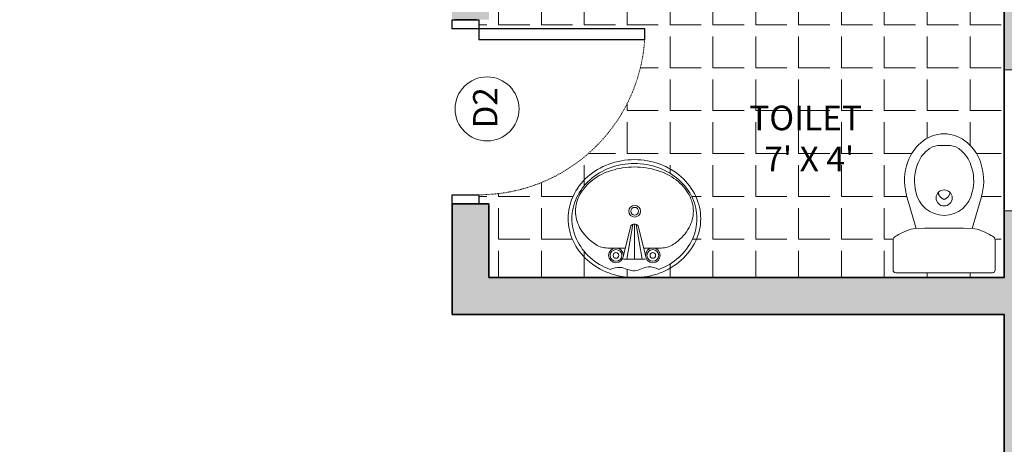
# Model space of a CAD drawing. Units: inches. Extents: x 2701 to 6846, y 811 to 2447.
# Tile 14 of 20: x 2926 to 3086, y 1231 to 1300. Entities that reach past the tile are written whole.
import ezdxf

# ---------------------------------------------------------------- set-up
doc = ezdxf.new("R2010")
doc.units = ezdxf.units.IN
doc.linetypes.add('HIDDEN4', pattern=[0.09375, 0.0625, -0.03125])
for name, color, linetype, lineweight in [('A-ANNO-IDEN', 7, 'Continuous', 13), ('A-AREA-IDEN', 7, 'Continuous', 18), ('A-DOOR', 4, 'Continuous', 25), ('A-DOOR-SWNG', 4, 'HIDDEN4', 13), ('A-FLOR-FIXT', 7, 'Continuous', 18), ('A-FLOR-PATT', 252, 'Continuous', 13), ('A-GLAZ', 4, 'Continuous', 18), ('A-WALL', 7, 'Continuous', 35)]:
    doc.layers.add(name, color=color, linetype=linetype, lineweight=lineweight)
doc.layers.add('A-WALL-PATT', color=18, linetype='Continuous', lineweight=13, true_color=0x000000)
doc.styles.get("Standard").update_dxf_attribs({"font": 'arial.ttf'})

# ---------------------------------------------------------------- blocks, each defined once
blk = doc.blocks.new('V')
for p, q in [((3304.149234297809, 1279.327014385662), (3281.149234297809, 1279.327014385662)), ((3304.149234297809, 1277.327014385662), (3281.149234297809, 1277.327014385662)), ((3304.149234297809, 1275.327014385662), (3281.149234297809, 1275.327014385662)), ((3281.149234297809, 1273.327014385662), (3304.149234297809, 1273.327014385662))]:
    blk.add_line(p, q)
blk.add_circle((3293.674463800009, 1283.693074863908), 3.189132293142032)
at = {"insert": (3292.450488040435, 1284.761898613762), "char_height": 2.5, "attachment_point": 1}
blk.add_mtext_dynamic_manual_height_columns('V', width=0.0152702913619578, gutter_width=12.5, heights=[0], dxfattribs=at)
blk = doc.blocks.new('V1')
for p, q in [((3281.149234297809, 1279.327014385662), (3281.149234297809, 1273.327014385662)), ((3304.149234297809, 1273.327014385662), (3304.149234297809, 1279.327014385662))]:
    blk.add_line(p, q)
blk.add_blockref('V', (0, 0))
blk = doc.blocks.new('A$C62EA08CE')
at = {"linetype": 'ByBlock'}
for p, q in [((0.2190750854661019, 0.3943350335612194), (0.306705085467911, 0.3943350335612194)), ((0.2328389724007138, 0.3943350335612194), (0.256592247476874, 0.2566437564746593)), ((0.2628900854706444, 0.3943350335612194), (0.2628900854706444, 0.2555161210839287)), ((0.2933077018988115, 0.3943350335612194), (0.2695802776597702, 0.256794098582759)), ((0.2190750854661019, 0.3797300335645559), (0.2482850854667049, 0.2628900335621438)), ((0.2774950854673079, 0.2628900335621438), (0.306705085467911, 0.3797300335645559)), ((0.1569030901755468, 0.3505200335639529), (0.2263775854680716, 0.3505200335639529)), ((0.2994025854659412, 0.3505200335639529), (0.3690778702966782, 0.3505200335639529))]:
    blk.add_line(p, q, dxfattribs=at)
for centre, radius in [((0.1898650854727748, 0.3797300335645559), 0.02921), ((0.1898650854727748, 0.3797300335645559), 0.02321), ((0.1898650854727748, 0.3797300335645559), 0.01121), ((0.335915085468514, 0.3797300335645559), 0.02921), ((0.335915085468514, 0.3797300335645559), 0.02321), ((0.335915085468514, 0.3797300335645559), 0.01121), ((0.2640384579517558, 0.2045255693010404), 0.023368), ((0.2640384579517558, 0.2045255693010404), 0.015368)]:
    blk.add_circle(centre, radius, dxfattribs=at)
for centre, radius, start, end in [((0.2518357941607974, 0.202225176646607), 0.2631644933429036, 110.2132031902237, 131.6335499305747), ((0.2518357941607974, 0.202225176646607), 0.2481644933429036, 110.2132031902237, 131.6335499305747), ((0.2628901093212335, 0.172201390065311), 0.2951586434963838, 90.00000458569829, 110.2131769401282), ((0.2628900616127794, 0.172201390065311), 0.2951586434963838, 69.78682305987175, 89.9999954143017), ((0.2739443767732155, 0.202225176646607), 0.2481644933429035, 48.36645006942531, 69.78679680977629), ((0.2739443767732155, 0.202225176646607), 0.2631644933429035, 48.36645006942531, 69.78679680977629), ((0.2348020259832992, 0.2213881285715615), 0.2375253048786466, 131.6335451873388, 155.0149376704166), ((0.2909781449579896, 0.2213881285715615), 0.2375253048786464, 24.98506232958336, 48.36645481266113), ((0.2348020259832992, 0.2213881285715615), 0.2225253048786466, 131.6335451873388, 155.0149376704166), ((0.2909781449579896, 0.2213881285715615), 0.2225253048786464, 24.98506232958336, 48.36645481266113), ((0.2084237233957538, 0.23368008415855), 0.208423637924446, 155.0149182782628, 180.0000137570949), ((0.2084237233957538, 0.23368008415855), 0.1934236379244461, 155.0149182782628, 180.0000137570949), ((0.2106628391502454, 0.177718259532412), 0.18834914705, 122.2598079089317, 151.0887990604045), ((0.1569030901755468, 0.2628900335621438), 0.08763, 90, 122.2598079089317), ((0.3690778702966782, 0.2628900335621438), 0.08763, 56.09549019404326, 90), ((0.2835224813406967, 0.1355918312110589), 0.24100718245, 53.1301018541481, 56.09549019404326), ((0.3151173317910434, 0.177718259532412), 0.18834914705, 28.91120093959547, 53.1301018541481), ((0.317356447545535, 0.23368008415855), 0.1934236379244455, 359.9999862429051, 24.98508172173719), ((0.317356447545535, 0.23368008415855), 0.2084236379244456, 359.9999862429051, 24.98508172173719), ((0.1622244803456851, 0.2044700335609377), 0.13301439488, 151.0887990604045, 180), ((0.2628900854706444, 0.2736666355558555), 0.018150514468869, 216.4225302188404, 323.5774697811596), ((0.3635556905883277, 0.2044700335609377), 0.13301439488, 0, 28.91120093959547), ((0.2084237233957538, 0.2336799829718075), 0.2084236379244456, 179.9999862429051, 204.9850817217372), ((0.2084237233957538, 0.2336799829718075), 0.1934236379244455, 179.9999862429051, 204.9850817217372), ((0.1622244803456851, 0.2044700335609377), 0.13301439488, 180, 208.9112009395955), ((0.3635556905883277, 0.2044700335609377), 0.13301439488, 331.0887990604045, 0), ((0.317356447545535, 0.2336799829718075), 0.1934236379244461, 335.0149182782628, 1.37570948859e-05), ((0.317356447545535, 0.2336799829718075), 0.208423637924446, 335.0149182782628, 1.37570948859e-05), ((0.2348020259832992, 0.2459719385587959), 0.2375253048786464, 204.9850623295834, 228.3664548126612), ((0.2348020259832992, 0.2459719385587959), 0.2225253048786464, 204.9850623295834, 228.3664548126612), ((0.2106628391502454, 0.2312218075967394), 0.18834914705, 208.9112009395955, 233.1301018541481), ((0.3151173317910434, 0.2312218075967394), 0.18834914705, 306.8698981458519, 331.0887990604045), ((0.2909781449579896, 0.2459719385587959), 0.2225253048786466, 311.6335451873388, 335.0149376704167), ((0.2909781449579896, 0.2459719385587959), 0.2375253048786466, 311.6335451873388, 335.0149376704167), ((0.2518357941607974, 0.2651348904837505), 0.2481644933429134, 228.3664500694253, 249.7867968097763), ((0.2422576896005921, 0.2733482359108166), 0.24100718245, 233.1301018541481, 252.7420607856108), ((0.2835224813406967, 0.2733482359108166), 0.24100718245, 287.2579392143892, 306.8698981458519), ((0.2739443767732155, 0.2651348904837505), 0.2481644933429136, 290.2132031902237, 311.6335499305747), ((0.2518357941607974, 0.2651348904837505), 0.2631644933429134, 228.3664500694253, 249.7867968097763), ((0.2628900854706444, 0.3397629544924712), 0.31055292093, 252.7420607856108, 270), ((0.2628900854706444, 0.3397629544924712), 0.31055292093, 270, 287.2579392143892), ((0.2739443767732155, 0.2651348904837505), 0.2631644933429136, 290.2132031902237, 311.6335499305747), ((0.2628901093212335, 0.2951586770577705), 0.2951586434963766, 249.7868230598717, 269.9999954143017), ((0.2628901093212335, 0.2951586770577705), 0.2801586434963766, 249.7868230598717, 269.9999954143017), ((0.2628900616127794, 0.2951586770577705), 0.2801586434963765, 270.0000045856983, 290.2131769401283), ((0.2628900616127794, 0.2951586770577705), 0.2951586434963765, 270.0000045856983, 290.2131769401283)]:
    blk.add_arc(centre, radius, start, end, dxfattribs=at)
blk.add_open_spline([(0.1660913743126002, 0.4351060694243643), (0.1795429390761559, 0.4305676737460202), (0.2123752678413389, 0.4194904420932696), (0.2631088802261481, 0.454314446693237), (0.3131553959096029, 0.4161820139975771), (0.3454695139184305, 0.4293234167515693), (0.3596887966214126, 0.4351060694243643)], degree=3, knots=[0, 0, 0, 0, 0.0411087303528805, 0.1003374234737184, 0.1559132068848227, 0.1995857666183122, 0.1995857666183122, 0.1995857666183122, 0.1995857666183122], dxfattribs=at)
blk = doc.blocks.new('A$C150B42AD')
at = {"ltscale": 20}
for p, q in [((0.2429999219411911, 0.6605010896237218), (0.0124999219360689, 0.6605010896237218)), ((0.2429999219411911, 0.6605010896237218), (0.4734999219390375, 0.6605010896237218)), ((-7.80610208e-08, 0.6480010896266322), (-7.80610208e-08, 0.5079979540751083)), ((0.4859999219361271, 0.6480010896266322), (0.4859999219361271, 0.5079979540751083)), ((0.1099663932354815, 0.4499086118448759), (0.0669662435202554, 0.3038111749119707)), ((0.1071200985052201, 0.4500080066427472), (0.1510932948976915, 0.4484724287904101)), ((0.1510932948976915, 0.4484724287904101), (0.2429999219411911, 0.4484724287904101)), ((0.3349065489774148, 0.4484724287904101), (0.2429999219411911, 0.4484724287904101)), ((0.3788797453698862, 0.4500080066427472), (0.3349065489774148, 0.4484724287904101)), ((0.3760334506469007, 0.4499086118448759), (0.419033600354851, 0.3038111749119707)), ((0.2244999219356032, 0.0549026304142899), (0.2429999219411911, 0.0549026304142899)), ((0.2614999219395031, 0.0549026304142899), (0.2429999219411911, 0.0549026304142899))]:
    blk.add_line(p, q, dxfattribs=at)
for centre, radius, start, end in [((0.0124999219360689, 0.6480010896266322), 0.0125, 90, 180), ((0.4734999219390375, 0.6480010896266322), 0.0125, 0, 90), ((0.0239999219365927, 0.5079979540751083), 0.024, 180, 243.9999999999169), ((0.2288323805723849, 0.861211124320107), 0.4322502624564528, 240.1180548737387, 247.8819451258213), ((0.2571674633099974, 0.861211124320107), 0.4322502624564528, 292.1180548741787, 299.8819451262613), ((0.4619999219385136, 0.5079979540751083), 0.024, 296.0000000000832, 0), ((0.1119175659141547, 0.5519209073245293), 0.1020257566424159, 243.3048371366711, 267.3048371363805), ((0.3740822779682276, 0.5519209073245293), 0.1020257566424159, 272.6951628636196, 296.6951628633288), ((0.2429999219411911, 0.2520000365038868), 0.1359999999999445, 90, 170.1093554438925), ((0.2429999219411911, 0.2520000365038868), 0.1359999999999054, 9.890644556107487, 90), ((0.2429999219411911, 0.3047433868632652), 0.0383668793900662, 90, 270), ((0.2429999219411911, 0.3047433868632652), 0.0383668793900662, 270, 90), ((0.3111168528876078, 0.2222454825459863), 0.2564589547706602, 165.7117968948095, 200.3376824053133), ((0.2429999219411911, 0.2520000365038868), 0.1834999999995578, 163.5995179369745, 169.4685073238174), ((0.2251027765405524, 0.2821865844234708), 0.0095725464836317, 149.1844377639907, 231.8077122469979), ((0.2644505607122483, 0.2649244167114375), 0.0524797911919514, 119.1738126186074, 155.015614861567), ((0.2438841986540865, 0.2978098350213258), 0.0138752344263254, 93.65396949145695, 111.1904535314196), ((0.2421156452282958, 0.2978098350213258), 0.0138752344263254, 68.80954646858042, 86.34603050854304), ((0.221549283162858, 0.2649244167114375), 0.0524797911919514, 24.98438513843297, 60.82618738139257), ((0.2608970673345539, 0.2821865844234708), 0.0095725464836317, 308.1922877530021, 30.81556223600924), ((0.1748829909874985, 0.2222454825459863), 0.2564589547707392, 339.6623175946867, 14.28820310476077), ((0.2429999219411911, 0.2520000365038868), 0.1834999999998773, 10.53149267661153, 16.40048206346955), ((0.3111168528876078, 0.2222454825459863), 0.2089589547707847, 165.2744742501726, 200.6077610261089), ((0.1748829909874985, 0.2222454825459863), 0.2089589547707847, 339.3922389738912, 14.72552574982734), ((0.2579999219406091, 0.1940000364993466), 0.1494999999998057, 197.6390904734559, 230.6281882087223), ((0.2279999219417732, 0.1940000364993466), 0.1494999999996299, 309.3718117912777, 342.360909526544), ((0.2579999219406091, 0.1940000364993466), 0.1969999999999626, 198.0034048038204, 230.2740437647753), ((0.2279999219417732, 0.1940000364993466), 0.1969999999999626, 309.7259562352247, 341.9965951961797), ((0.2429999219411911, 0.1660000365009182), 0.1184999999993879, 227.6454679706322, 235.8467474759224), ((0.2244999219356032, 0.149902630415454), 0.0949999999999961, 239.6323803004523, 270), ((0.2614999219395031, 0.149902630415454), 0.0949999999999961, 270, 300.3676196995477), ((0.2429999219411911, 0.1660000365009182), 0.1185000000000767, 304.1532525240776, 312.3545320293678), ((0.2429999219411911, 0.1660000365009182), 0.1660000000001673, 228.0788004750028, 270), ((0.2429999219411911, 0.1660000365009182), 0.16599999999994, 270, 311.9211995251523)]:
    blk.add_arc(centre, radius, start, end, dxfattribs=at)
blk = doc.blocks.new('DOOR-D2-30IN-PANEL-FRAME')
blk.add_lwpolyline([(-4.547e-13, 30.00000000000046), (-4.547e-13, 28.52062868157645), (4.3614931230818, 28.52062868157645), (4.3614931230818, 30.00000000000046), (-4.547e-13, 30.00000000000046)], close=True)
for points in [[(3.925343810773938, 30.00000000000046), (0.4361493129576957, 30.00000000000046)], [(4.361493123406944, 0), (4.361493123406944, 3.223968567697738), (31.40275048651847, 3.22396856790101), (31.40275048651847, 1.479371318667745), (1.623448e-10, 1.479371318424), (1.623448e-10, 0)], [(1.623448e-10, 0), (4.361493123406944, 0)], [(3.925343810773938, 0), (0.4361493129576957, 0)]]:
    blk.add_lwpolyline(points)

msp = doc.modelspace()

# ---------------------------------------------------------------- hatches: boundary and pattern name
at = {"layer": 'A-FLOR-PATT'}
h = msp.add_hatch(dxfattribs=at)
h.set_pattern_fill('ANGLE', color=256)
h.set_pattern_definition([(0, (0, 0), (0, 6.985), [5.08, -1.905]), (90, (0, 0), (-6.985, 4e-16), [5.08, -1.905])])
h.paths.add_polyline_path([(2841.812531618507, 1296.510714093028, -0.1094531397224823), (2842.614165366529, 1300.128842847245, -0.1023747835315324), (2844.977063233859, 1303.301704019213, -0.0937428406070795), (2848.425874088265, 1305.367635711971, -0.0624630522953803), (2851.366818664733, 1306.050044742079), (2785.971391037217, 1306.050044742079), (2785.971391037217, 1258.050044742079), (2827.971391037217, 1258.050044742079), (2827.971391037217, 1256.411537864998), (2829.450762355621, 1256.411537864998, -0.3948265708167148), (2854.747422469505, 1283.452795228435), (2856.49201971855, 1283.452795228435), (2856.49201971876, 1256.411537865324), (2857.971391037219, 1256.411537865324), (2857.971391037219, 1258.05004474208), (2863.971391037218, 1258.050044742079), (2863.971391037217, 1306.050044742079), (2853.867060923166, 1306.050044742079, -0.0624630504647152), (2856.808005416599, 1305.367635742541, -0.0937428427235612), (2860.256816355725, 1303.301704017657, -0.1023747714125829), (2862.619714024758, 1300.128843269809, -0.1094531521575188), (2863.421347969692, 1296.510714138194, -0.109453153989093), (2862.619714017641, 1292.892584946142, -0.1023747709767553), (2860.256816355757, 1289.719724213534, -0.093738257087872), (2856.808189965141, 1287.653860434733, -0.0884250558281599), (2852.616939784454, 1286.906795737127, -0.0884250554332989), (2848.425689622791, 1287.653860434813, -0.0937382570330623), (2844.977063234018, 1289.719724212192, -0.1023747824199799), (2842.614165384649, 1292.892585345091, -0.1094531396555831)])
h.paths.add_polyline_path([(2805.214857085719, 1273.877134568363, -0.141745245190178), (2808.318689175414, 1271.772621468736, -0.1849834247598648), (2809.773740825251, 1267.974277286972, -0.1849834247688995), (2808.318689175285, 1264.175933105053, -0.141745244968364), (2805.214857091107, 1262.071420007333, -0.1522440861962393), (2799.994488829542, 1261.79557176336, -0.0256138964539793), (2799.368711507224, 1261.94541476925), (2794.365115778627, 1263.418098821323), (2794.36467071784, 1263.405353947873, -0.1112416791490392), (2793.99312620013, 1261.915170284834, -0.0338893268367682), (2793.114424873909, 1260.113565580275, -0.286745385218), (2792.375651823606, 1259.651928944151), (2787.580775843661, 1259.651928944133, -0.4142135623681101), (2787.152671505053, 1260.080033282747), (2787.152671505153, 1267.974277286972), (2787.152671505053, 1275.868521290948, -0.4142135623730951), (2787.580775843668, 1276.296625629562), (2792.375651823623, 1276.296625629544, -0.2867453846084762), (2793.114424873105, 1275.834988995069, -0.0338893268640583), (2793.99312620013, 1274.033384289111, -0.1051042356073151), (2794.361711671137, 1272.627936636842), (2794.365115778619, 1272.530455752619), (2799.368711507498, 1274.003139804786, -0.0256138965941945), (2799.994488833287, 1274.152982811292, -0.1522440859162748)], flags=16)
h.paths.add_polyline_path([(2804.681063364808, 1272.339952816459, -0.1449445299175104), (2807.087654609562, 1270.708506585421, -0.0358001151589041), (2807.447023191777, 1270.252713401882, -0.1332846890906797), (2807.893417732773, 1268.607871708063), (2807.893417732813, 1267.974277286972), (2807.893417732773, 1267.340682865632, -0.1332846888970446), (2807.447023193029, 1265.695841173949, -0.0358001152638917), (2807.087654609923, 1265.240047988954, -0.1449445297267833), (2804.681063368992, 1263.608601758809, -0.1554037438169349), (2800.343099481134, 1263.385728797012, -0.3645106918446579), (2796.485382154562, 1267.974277286972, -0.3645106920174053), (2800.343099483932, 1272.562825777418, -0.1554037435534987)], flags=0)
h.paths.add_polyline_path([(2800.015880108981, 1268.901471623875, 0.1692977046764319), (2799.131174998024, 1268.11576383613, 0.0766670309700064), (2799.100009657075, 1267.974277286936, 0.0766670313951798), (2799.13117499834, 1267.832790736999, 0.1692977045836763), (2800.015880108981, 1267.04708294982, 0.3052192884941762), (2800.365297210358, 1267.156497374013, 0.1695347489604994), (2800.650786991011, 1267.974277286972, 0.1695347391656343), (2800.365297241503, 1268.792057160761, 0.3052193300480048)], flags=0)
h.paths.add_polyline_path([(2971.971391037218, 1456.050044742079), (2923.971391037218, 1456.050044742079), (2923.971391037218, 1408.050044742079), (2922.332884160136, 1408.050044742079), (2922.332884160136, 1406.570673423676, -0.394826570816717), (2949.374141523573, 1381.274013309792), (2949.374141523573, 1379.529416060747), (2922.332884160461, 1379.529416060537), (2922.332884160461, 1378.050044742079), (2923.971391037218, 1378.050044742079), (2923.971391037217, 1372.050044742079), (2971.971391037217, 1372.050044742079)])
h.paths.add_polyline_path([(2939.8177624336, 1436.526417411941, -0.1417452451905352), (2937.713249333971, 1433.422585322236, -0.1849834247599418), (2933.914905152205, 1431.967533672398, -0.1849834247691276), (2930.116560970283, 1433.422585322367, -0.1417452449676952), (2928.01204787257, 1436.526417406529, -0.1522440861964963), (2927.736199628592, 1441.746785668103, -0.0256138964540868), (2927.886042634483, 1442.372562990423), (2929.358726686557, 1447.376158719022), (2929.345981813088, 1447.376603779809, -0.1112416791473441), (2927.855798150072, 1447.748148297517, -0.0338893268369074), (2926.054193445506, 1448.626849623741, -0.2867453852169366), (2925.592556809384, 1449.365622674043), (2925.592556809366, 1454.160498653989, -0.4142135623681173), (2926.020661147981, 1454.588602992596), (2933.914905152205, 1454.588602992496), (2941.809149156182, 1454.588602992596, -0.4142072303161659), (2942.237253494696, 1454.160507909187), (2942.237253494777, 1449.365622674043, -0.2867453846243844), (2941.775616860276, 1448.626849624529, -0.0338893268635044), (2939.974012154347, 1447.74814829752, -0.1051042356087532), (2938.568564502058, 1447.379562826511), (2938.471083617852, 1447.37615871903), (2939.943767670019, 1442.372562990154, -0.0256138965942444), (2940.093610676525, 1441.746785664364, -0.152244085915992)], flags=16)
h.paths.add_polyline_path([(2938.280580681695, 1437.060211132847, -0.1449445299182329), (2936.649134450649, 1434.653619888082, -0.0358001151583613), (2936.193341267117, 1434.294251305872, -0.1332846890907526), (2934.548499573297, 1433.847856764876), (2933.914905152205, 1433.847856764836), (2933.281310730865, 1433.847856764876, -0.1332846888976268), (2931.636469039176, 1434.294251304624, -0.0358001152630847), (2931.180675854191, 1434.653619887722, -0.14494452972667), (2929.549229624045, 1437.06021112865, -0.1554037438170702), (2929.326356662246, 1441.398175016512, -0.3645106918448713), (2933.914905152205, 1445.255892343087, -0.3645106920173691), (2938.503453642651, 1441.398175013717, -0.1554037435532691)], flags=0)
h.paths.add_polyline_path([(2969.158462562638, 1392.044508285666, -0.0937428443921736), (2971.224394311477, 1388.595697278927, -0.0884209696484748), (2971.971391037217, 1384.404631716083, -0.0884209680179829), (2971.224394332037, 1380.213566228077, -0.0937428458331012), (2969.158462561081, 1376.764755163806, -0.1023747798731684), (2965.985601516888, 1374.401857356678, -0.1094531425013952), (2962.367472681615, 1373.600223549837, -0.1094531553411192), (2958.74934344807, 1374.401857521223, -0.102374769792102), (2955.576482756955, 1376.764755163771, -0.0937382570879047), (2953.510618978154, 1380.213381554388, -0.0884250558281564), (2952.763554280548, 1384.404631735075, -0.0884250554336261), (2953.510618978239, 1388.595881896752, -0.0937382570324601), (2955.576482755607, 1392.044508285504, -0.1023747638736991), (2958.749343238892, 1394.40740583216, -0.10945316082308), (2962.367472636449, 1395.209039901022, -0.1094531494878097), (2965.985601690358, 1394.407406013345, -0.102374774975509)], flags=0)
edge = h.paths.add_edge_path(flags=16)
edge.add_arc((2961.074722408913, 1384.858947505427), 10.19921062335061, 20.21320321302568, 41.63359467655653, ccw=False)
edge.add_spline(control_points=[(2970.645798607602, 1388.382922212802), (2970.45927694694, 1387.830081875375), (2970.004018351208, 1386.480719475378), (2971.435235818619, 1384.395639569603), (2969.86804662324, 1382.338798369057), (2970.408139739579, 1381.010733700175), (2970.645798607602, 1380.426341238356)], knot_values=[0, 0, 0, 0, 0.0411087303528805, 0.1003374234737184, 0.1559132068848227, 0.1995857666183122, 0.1995857666183122, 0.1995857666183122, 0.1995857666183122], degree=3, periodic=0)
edge.add_arc((2961.074722408954, 1383.950315945844), 10.19921062335061, 318.3664053106646, 339.7867967863075, ccw=False)
edge.add_arc((2961.862292702369, 1383.250252100635), 9.145476143303874, 294.98529005245234, 318.3664053112933, ccw=False)
edge.add_arc((2962.367474738348, 1382.166141072693), 7.949438681384353, 269.9999862429006, 294.9853451035073, ccw=False)
edge.add_arc((2962.367470579714, 1382.166141072693), 7.949438681384465, 245.0146528606722, 270.00001621636034, ccw=False)
edge.add_arc((2962.872652615592, 1383.250252100682), 9.145476143303885, 221.633594689284, 245.0147081786685, ccw=False)
edge.add_arc((2963.660222908995, 1383.950315945905), 10.19921062335051, 200.2129623510071, 221.6335946899624, ccw=False)
edge.add_arc((2964.894158186733, 1384.404632705954), 11.5141250647146, 180.0000045856949, 200.2129623497761, ccw=False)
edge.add_arc((2964.894158186734, 1384.404630744956), 11.51412506471477, 159.7870376490639, 179.999994827515, ccw=False)
edge.add_arc((2963.660222908922, 1384.858947504804), 10.19921062335051, 138.3664053200289, 159.7870376464858, ccw=False)
edge.add_arc((2962.872652615694, 1385.559011350224), 9.145476143303881, 114.9852895697228, 138.3664053235114, ccw=False)
edge.add_arc((2962.367470579715, 1386.643122378167), 7.949438681384341, 89.99998624290072, 114.9853445481478, ccw=False)
edge.add_arc((2962.367474738348, 1386.643122378167), 7.949438681384461, 65.01465414332972, 90.00001621635698, ccw=False)
edge.add_arc((2961.862292702924, 1385.559011349966), 9.145476143303876, 41.63359468007258, 65.01470929671348, ccw=False)
h.paths.add_polyline_path([(2963.809881193461, 1393.327235568244, -0.1264579126559968), (2966.613496696745, 1390.682864813822, -0.1416969839114421), (2967.169431848072, 1388.76054773013), (2967.169431848171, 1387.405856218539, -1), (2969.570411442753, 1387.40585621857, -0.4142135626407067), (2968.369921644365, 1386.205366421279), (2963.567962456663, 1385.004876624353, 0.146217798515541), (2963.311249278865, 1384.663463983469), (2968.97016654397, 1385.639690083447), (2968.97016654397, 1383.154510596366), (2963.317428127216, 1384.129674263443, 0.1403115373898127), (2963.56796245605, 1383.804386826958), (2968.369921645561, 1382.603897029581, -0.4142135623489124), (2969.570411442753, 1381.403407232289, -1), (2967.169431848171, 1381.403407232289), (2967.169431848072, 1380.040463554169, -0.1490250791000606), (2966.557068512987, 1378.031526062613, -0.0127594246128423), (2966.264512020975, 1377.619349736432, -0.1063032105074506), (2963.809880694587, 1375.482028786924, -0.1268223860120219), (2961.166982861567, 1374.800713347196, -0.12682239841106), (2958.52408452876, 1375.482027883284, -0.1063031789236789), (2956.069454414507, 1377.619348785205, -0.0857220920089208), (2954.537253221299, 1380.622635309784, -0.0753510219692474), (2953.964044077883, 1384.404631725429, -0.0753510220208753), (2954.537253222076, 1388.186628143578, -0.0857220919249397), (2956.069454414099, 1391.189914665108, -0.1063031717113424), (2958.5240850283, 1393.327234664099, -0.1268223860250843), (2961.166982861567, 1394.008550103962, -0.1268223983642548)], flags=0)
h.paths.add_polyline_path([(2934.842099489099, 1441.725394388693, 0.1692977046741335), (2934.056391701355, 1442.610099499628, 0.0766670309649834), (2933.91490515217, 1442.641264840574, 0.0766670314095982), (2933.773418602207, 1442.610099499295, 0.1692977045780331), (2932.987710815057, 1441.72539438868, 0.305219290057435), (2933.097125240708, 1441.375977286128, 0.169534748594888), (2933.914905152205, 1441.090487506638, 0.1695347390414705), (2934.732685025499, 1441.375977255749, 0.3052193305973386)], flags=0)
h.paths.add_polyline_path([(2969.323819906164, 1387.40585621857, -1), (2967.416023384759, 1387.40585621857, -1)], flags=0)
h.paths.add_polyline_path([(2968.830636832988, 1387.40585621857, -1), (2967.909206457936, 1387.40585621857, -1)], flags=0)
h.paths.add_polyline_path([(2962.129657139981, 1384.357435236314, -1), (2960.208873464314, 1384.357435236314, -1)], flags=0)
h.paths.add_polyline_path([(2961.800868424529, 1384.357435236314, -1), (2960.537662179766, 1384.357435236314, -1)], flags=0)
h.paths.add_polyline_path([(2969.323819906164, 1381.403407232289, -1), (2967.416023384759, 1381.403407232289, -1)], flags=0)
h.paths.add_polyline_path([(2968.830636832988, 1381.403407232289, -1), (2967.909206457936, 1381.403407232289, -1)], flags=0)
h.paths.add_polyline_path([(3085.971391037217, 1306.050044742079), (3001.971391037217, 1306.050044742079), (3001.971391037217, 1300.050044742079), (3000.332884160462, 1300.050044742079), (3000.332884160462, 1298.570673423621), (3027.374141523574, 1298.570673423411), (3027.374141523574, 1296.826076174374, -0.3948265708167921), (3000.332884160137, 1271.529416060482), (3000.332884160137, 1270.050044742079), (3001.971391037216, 1270.050044742079), (3001.971391037217, 1258.050044742079), (3085.971391037217, 1258.050044742079)])
h.paths.add_polyline_path([(3033.332715044416, 1274.444953022308, -0.1023747723857111), (3035.695612729331, 1271.272092240373, -0.1094531510467398), (3036.49724665838, 1267.653963142847, -0.109453129065687), (3035.695613062762, 1264.035834715682, -0.102374792813879), (3033.332715044451, 1260.862973218194, -0.0937428491083937), (3029.883903848349, 1258.797041398739, -0.0884209654955001), (3025.692838473141, 1258.05004474208, -0.0884209669723455), (3021.501773032378, 1258.797041429867, -0.093742846952782), (3018.052961922706, 1260.862973216846, -0.1023747779170817), (3015.690064146835, 1264.035834192024, -0.1094531447948728), (3014.888430307195, 1267.653963097683, -0.1094531229044609), (3015.690063814699, 1271.272091335764, -0.1023747982671114), (3018.052961922546, 1274.444953023867, -0.0937382570344717), (3021.501588311451, 1276.510816801145, -0.0884250558280669), (3025.692838492134, 1277.25788149875, -0.0884250554332868), (3029.884088653796, 1276.510816801064, -0.0937382570874262)], flags=0)
edge = h.paths.add_edge_path(flags=16)
edge.add_arc((3026.847218107582, 1267.148783163603), 9.145476143303444, 24.985288685417686, 48.36640531129461, ccw=False)
edge.add_arc((3027.931329135525, 1267.653965199581), 7.949438681383711, -1.3757099395661498e-05, 24.98534353079839, ccw=False)
edge.add_arc((3027.931329135525, 1267.653961040948), 7.949438681383458, -24.98534255728248, 1.6216352207720774e-05, ccw=False)
edge.add_arc((3026.847218107536, 1268.159143076827), 9.145476143303622, 311.6335946892918, 335.0147121614734, ccw=False)
edge.add_arc((3026.147154262487, 1268.946713370386), 10.19921062335084, 290.21320321300624, 311.633594688656, ccw=False)
edge.add_spline(control_points=[(3029.671128969861, 1259.375637171695), (3029.086736508042, 1259.613296039718), (3027.758671839159, 1260.153389156057), (3025.701830638613, 1258.586199960678), (3023.616750732838, 1260.01741742809), (3022.267388332841, 1259.562158832357), (3021.714547995414, 1259.375637171695)], knot_values=[0, 0, 0, 0, 0.0436725597334895, 0.0992483431445938, 0.1584770362654316, 0.1995857666183122, 0.1995857666183122, 0.1995857666183122, 0.1995857666183122], degree=3, periodic=0)
edge.add_arc((3025.238522703413, 1268.946713370155), 10.19921062335076, 228.3664053199745, 249.78679678323948, ccw=False)
edge.add_arc((3024.538458857992, 1268.159143076927), 9.145476143303437, 204.9852869984493, 228.3664053234469, ccw=False)
edge.add_arc((3023.45434783005, 1267.65396104095), 7.949438681383719, 179.9999862429023, 204.9853415900221, ccw=False)
edge.add_arc((3023.454347830049, 1267.653965199583), 7.949438681383464, 155.0146544340279, 180.0000162163587, ccw=False)
edge.add_arc((3024.538458858251, 1267.148783164158), 9.14547614330361, 131.6335946800857, 155.0147095493943, ccw=False)
edge.add_arc((3025.238522702964, 1266.361212870303), 10.19921062335009, 110.2129623509966, 131.6335946778856, ccw=False)
edge.add_arc((3025.692839463013, 1265.127277592565), 11.51412506471423, 90.00000458569599, 110.2129623497689, ccw=False)
edge.add_arc((3025.692837502014, 1265.127277592564), 11.51412506471427, 69.78703764905441, 89.99999482750928, ccw=False)
edge.add_arc((3026.147154262372, 1266.361212870188), 10.19921062335108, 48.3664053106545, 69.78703764952758, ccw=False)
h.paths.add_polyline_path([(3032.478121424384, 1273.951981363762, -0.1063031716151077), (3034.615441420988, 1271.497350751304, -0.1268223860413822), (3035.296756861021, 1268.85445291773, -0.1268223983836015), (3034.615442325363, 1266.211554585404, -0.1063032176830601), (3032.478120473694, 1263.756923759752, -0.012759424397259), (3032.06594390682, 1263.464367621596, -0.1490250698458729), (3030.057006653981, 1262.852003931225), (3028.694062975896, 1262.852003931126, -0.4142135623806731), (3029.894552773218, 1261.651514133835, -1), (3027.493573178635, 1261.651514133737), (3026.293083381258, 1266.453473323247, 0.1403115373895235), (3025.967795944775, 1266.704007652081), (3026.94295961185, 1261.051269235327), (3024.457780124769, 1261.051269235327), (3025.434006224748, 1266.710186500432, 0.1462177985154153), (3025.092593583864, 1266.453473322634), (3023.892103786938, 1261.651514134932, -1.000000100073327), (3021.491124192355, 1261.651514133836, -0.4142135623731147), (3022.691613989647, 1262.852003931127), (3021.336922478021, 1262.852003931226, -0.1416970043012063), (3019.41460486282, 1263.407938240376, -0.1264579123471447), (3016.770235543815, 1266.211555085013, -0.1268223859959933), (3016.088920104255, 1268.854452917731, -0.1268223983918172), (3016.770234640404, 1271.497351250108, -0.1063031789240722), (3018.907555542179, 1273.951981364503, -0.0857220919129331), (3021.910842063079, 1275.484182556737, -0.0753510220530541), (3025.692838482788, 1276.057391701414, -0.075351022008823), (3029.474834900351, 1275.484182557402, -0.0857220920013936)], flags=0)
h.paths.add_polyline_path([(3072.364663406136, 1280.00178826655, -0.1849834247682267), (3076.163007588042, 1281.456839916512, -0.1849834247587431), (3079.961351769785, 1280.001788266685, -0.1417452451922909), (3082.065864869442, 1276.897956176945, -0.1522440859149591), (3082.341713112365, 1271.677587924556, -0.0256138965949624), (3082.191870105855, 1271.051810598748), (3080.719186053688, 1266.048214869872), (3080.816666937894, 1266.04481076239, -0.1051042356089094), (3082.222114590184, 1265.676225291381, -0.0338893268638024), (3084.023719296129, 1264.797523964363, -0.2867453846178035), (3084.485355930614, 1264.058750914859), (3084.485355930532, 1259.26388419012, -0.4142198944533688), (3084.057251592018, 1258.835770596306), (3076.163007588042, 1258.835770596406), (3068.268763583817, 1258.835770596306, -0.4142135623730951), (3067.840659245203, 1259.26387493492), (3067.84065924522, 1264.058750914876, -0.2867453852273427), (3068.302295881383, 1264.797523965184, -0.0338893268359893), (3070.103900585901, 1265.676225291382, -0.1051042356607345), (3071.509348238908, 1266.044810762424), (3071.606829122393, 1266.04821486988), (3070.134145070319, 1271.051810598479, -0.0256138964541135), (3069.984302064428, 1271.6775879208, -0.1522440861962023), (3070.260150308403, 1276.897956182364, -0.1417452449689107)], flags=16)
h.paths.add_polyline_path([(3073.428778290028, 1278.770753701179, -0.0358001152649927), (3073.884571475038, 1279.130122284293, -0.1332846888953009), (3075.529413166701, 1279.576516824026), (3076.163007588042, 1279.576516824066), (3076.796602009133, 1279.576516824026, -0.1332846890885353), (3078.441443702929, 1279.130122283046, -0.0358001151610664), (3078.897236886497, 1278.77075370081, -0.1449445299169966), (3080.528683117528, 1276.364162456064, -0.1554037435538929), (3080.751556078487, 1272.026198575177, -0.3645106920168784), (3076.163007588042, 1268.168481245816, -0.3645106918444272), (3071.574459098083, 1272.026198572385, -0.1554037438173037), (3071.797332059881, 1276.364162460253, -0.1449445297265802)], flags=0)
h.paths.add_polyline_path([(3026.700426809735, 1268.85217047715, -1), (3024.77964313407, 1268.85217047715, -1)], flags=0)
h.paths.add_polyline_path([(3026.371638094284, 1268.85217047715, -1), (3025.108431849521, 1268.85217047715, -1)], flags=0)
h.paths.add_polyline_path([(3075.268500788244, 1271.624470471877, 0.1576769337924287), (3076.021521038093, 1270.814274089584, 0.0766670314188588), (3076.163007588078, 1270.783108748328, 0.0766670308737057), (3076.3044941371, 1270.814274089222, 0.1576769338966524), (3077.057514387587, 1271.624470471873, 0.3746263233786361), (3076.980787467475, 1272.048396328269, 0.1695347405768383), (3076.163007588042, 1272.333886082264, 0.1695347491173554), (3075.345227674456, 1272.04839630111, 0.3746262855823952)], flags=0)
h.paths.add_polyline_path([(3029.64796123663, 1261.651514133835, -1), (3027.740164715224, 1261.651514133835, -1)], flags=0)
h.paths.add_polyline_path([(3029.154778163453, 1261.651514133835, -1), (3028.233347788401, 1261.651514133835, -1)], flags=0)
h.paths.add_polyline_path([(3023.645512250349, 1261.651514133836, -1), (3021.737715728944, 1261.651514133836, -1)], flags=0)
h.paths.add_polyline_path([(3023.152329177172, 1261.651514133836, -1), (3022.23089880212, 1261.651514133836, -1)], flags=0)
h.paths.add_polyline_path([(2810.572659831725, 1281.221625132062), (2833.310943898055, 1281.221625132062), (2833.310943898055, 1296.429027198873), (2810.572659831725, 1296.429027198873)], flags=24)
h.paths.add_polyline_path([(2937.545180300932, 1410.244315705433), (2960.208482391776, 1410.244315705433), (2960.208482391776, 1425.451717772244), (2937.545180300932, 1425.451717772244)], flags=24)
h.paths.add_polyline_path([(3043.227580059905, 1273.098575462184), (3065.890882150748, 1273.098575462184), (3065.890882150748, 1288.305977528995), (3043.227580059905, 1288.305977528995)], flags=24)
at = {"layer": 'A-WALL-PATT'}
h = msp.add_hatch(color=256, dxfattribs=at)
h.dxf.hatch_style = 1
h.paths.add_polyline_path([(3085.971391037218, 1456.050044742079), (3085.971391037217, 1348.050044742079), (3091.971391037218, 1348.050044742079), (3091.971391037218, 1360.050044742079), (3091.971391037218, 1462.050044742079), (2960.086244240269, 1462.050044742079), (2960.086244240269, 1456.050044742079), (2971.971391037218, 1456.050044742079), (2971.971391037217, 1372.050044742079), (2923.971391037217, 1372.050044742079), (2923.971391037218, 1378.050044742079), (2917.971391037217, 1378.050044742079), (2917.971391037217, 1351.050044742079), (2923.971391037218, 1351.050044742079), (2923.971391037217, 1366.050044742079), (2971.971391037218, 1366.050044742079), (2971.971391037218, 1351.05004474208), (2976.76903347243, 1351.05004474208), (2977.971391037218, 1351.050044742079), (2977.971391037218, 1456.050044742079)])
h.paths.add_polyline_path([(2779.971391037218, 1462.050044742079), (2779.971391037218, 1342.05004474208), (2785.971391037217, 1342.05004474208), (2785.971391037218, 1456.050044742079), (2917.971391037218, 1456.050044742079), (2917.971391037217, 1408.050044742079), (2922.332884160136, 1408.050044742079), (2923.971391037218, 1408.050044742079), (2923.971391037218, 1456.050044742079), (2937.086244240269, 1456.050044742079), (2937.086244240269, 1462.050044742079)])
h.paths.add_polyline_path([(2779.971391037217, 1306.050044742079), (2779.971391037217, 1294.241199564278), (2785.971391037217, 1294.241199564278), (2785.971391037217, 1306.050044742079), (2851.366818664733, 1306.050044742079, -0.0258153414615714), (2852.616939803445, 1306.114632493797, -0.0258153410699148), (2853.867060923166, 1306.050044742079), (2863.971391037217, 1306.050044742079), (2863.971391037218, 1258.050044742079), (2857.971391037219, 1258.05004474208), (2857.971391037218, 1252.050044742079), (2878.971391037217, 1252.050044742079), (2878.971391037217, 1258.050044742079), (2869.971391037218, 1258.050044742079), (2869.971391037217, 1306.050044742079), (2923.971391037217, 1306.050044742079), (2923.971391037218, 1318.050044742079), (2919.173748601648, 1318.050044742079), (2917.971391037216, 1318.050044742079), (2917.971391037216, 1312.050044742079), (2785.971391037217, 1312.050044742079), (2785.971391037217, 1318.050044742079), (2779.971391037217, 1318.050044742079)])
h.paths.add_polyline_path([(2785.971391037218, 1252.050044742079), (2827.971391037217, 1252.050044742079), (2827.971391037217, 1256.411537864998), (2827.971391037217, 1258.050044742079), (2785.971391037217, 1258.050044742079), (2785.971391037217, 1271.241199564278), (2779.971391037218, 1271.241199564278), (2779.971391037218, 1174.050044742079), (2785.971391037217, 1174.050044742079)])
h.paths.add_polyline_path([(2779.971391037218, 1030.050044742079), (2869.971391037218, 1030.050044742079), (2869.971391037218, 1036.050044742079), (2785.971391037218, 1036.050044742079), (2785.971391037217, 1126.050044742079), (2917.971391037217, 1126.050044742079), (2917.971391037216, 1120.050044742079), (2923.971391037218, 1120.050044742078), (2923.971391037218, 1258.050044742079), (2911.971391037217, 1258.050044742079), (2911.971391037217, 1253.252402306509), (2911.971391037218, 1252.050044742079), (2917.971391037218, 1252.050044742079), (2917.971391037217, 1132.050044742078), (2785.971391037217, 1132.050044742079), (2785.971391037217, 1144.050044742079), (2779.971391037218, 1144.050044742079)])
h.paths.add_polyline_path([(2935.971391037218, 1030.050044742079), (2935.971391037218, 1033.050044742079), (2935.971391037217, 1036.050044742079), (2923.971391037218, 1036.050044742079), (2923.971391037218, 1087.050044742077), (2919.173748602005, 1087.050044742077), (2917.971391037216, 1087.050044742079), (2917.971391037218, 1036.050044742079), (2893.971391037218, 1036.050044742079), (2893.971391037218, 1030.050044742079)])
h.paths.add_polyline_path([(2971.971391037218, 1036.050044742079), (2971.971391037218, 1030.050044742079), (3091.971391037218, 1030.050044742079), (3091.971391037218, 1060.050044742079), (3085.971391037217, 1060.050044742079), (3085.971391037217, 1036.050044742079)])
h.paths.add_polyline_path([(3085.971391037217, 1084.050044742079), (3091.971391037217, 1084.050044742079), (3091.971391037217, 1096.050044742079), (3091.971391037217, 1268.891476913671), (3085.971391037217, 1268.891476913671), (3085.971391037217, 1258.050044742079), (3001.971391037217, 1258.050044742079), (3001.971391037216, 1270.050044742079), (2995.971391037217, 1270.050044742079), (2995.971391037217, 1252.050044742079), (3085.971391037217, 1252.050044742079)])
h.paths.add_polyline_path([(3085.971391037217, 1306.050044742078), (3085.971391037217, 1291.891476913671), (3091.971391037218, 1291.891476913671), (3091.971391037218, 1318.050044742079), (3085.971391037217, 1318.050044742079), (3085.971391037217, 1312.050044742079), (2977.971391037218, 1312.050044742079), (2977.971391037217, 1318.050044742079), (2971.971391037218, 1318.050044742079), (2971.971391037218, 1306.050044742079), (2995.971391037217, 1306.050044742079), (2995.971391037217, 1300.050044742079), (3000.332884160462, 1300.050044742079), (3001.971391037217, 1300.050044742079), (3001.971391037217, 1306.050044742079)])

# ---------------------------------------------------------------- linework, layer by layer
at = {"layer": 'A-ANNO-IDEN'}
msp.add_circle((3001.681908773835, 1285.517126868154), 5.217112562990953, dxfattribs=at)
at = {"layer": 'A-DOOR-SWNG'}
msp.add_arc((3000.332884160462, 1298.630831949429), 27.10141588894677, 270, 356.1816951334161, dxfattribs=at)
at = {"layer": 'A-WALL'}
for p, q in [((3085.971391037217, 1306.050044742079), (3085.971391037217, 1258.050044742079)), ((3001.971391037216, 1270.050044742079), (2995.971391037217, 1270.050044742079)), ((2995.971391037217, 1270.050044742079), (2995.971391037217, 1252.050044742079)), ((3001.971391037216, 1270.050044742079), (3001.971391037217, 1258.050044742079)), ((3085.971391037217, 1258.050044742079), (3001.971391037217, 1258.050044742079)), ((3085.971391037219, 1252.050044742079), (2995.971391037217, 1252.050044742079)), ((3085.971391037217, 1252.050044742079), (3085.971391037217, 1056.050044742079))]:
    msp.add_line(p, q, dxfattribs=at)

# ---------------------------------------------------------------- block references
at = {"layer": 'A-DOOR', "extrusion": (0, 0, -1), "zscale": -1, "rotation": 180}
msp.add_blockref('DOOR-D2-30IN-PANEL-FRAME', (-2995.971391037055, 1300.050044742077), dxfattribs=at)
at = {"layer": 'A-FLOR-FIXT'}
for name, p, xscale, yscale, zscale, rotation in [('A$C150B42AD', (3067.840661918763, 1281.456841166602), -34.24834708915159, 34.24834708915159, 34.24834708915159, 180), ('A$C62EA08CE', (3014.888426794445, 1277.257882878076), -41.09858943139644, 41.09858943139644, 41.09858943139644, 179.9999999999955)]:
    msp.add_blockref(name, p, dxfattribs=dict(at, xscale=xscale, yscale=yscale, zscale=zscale, rotation=rotation))
at = {"layer": 'A-GLAZ', "rotation": 270}
msp.add_blockref('V1', (1812.644376651556, 4573.040711211481), dxfattribs=at)

# ---------------------------------------------------------------- texts
at = {"layer": 'A-ANNO-IDEN', "insert": (3003.370646027497, 1282.327041569554), "char_height": 3.968122321300642, "attachment_point": 7, "rotation": 90.00000000000001}
msp.add_mtext_dynamic_manual_height_columns('D2', width=1.694637290736917, gutter_width=49.60152901625804, heights=[0], dxfattribs=at)
at = {"layer": 'A-AREA-IDEN', "insert": (3044.406383232219, 1286.042819634259), "char_height": 4, "attachment_point": 1}
msp.add_mtext_dynamic_manual_height_columns("{\\fTimes New Roman|b0|i0|c0|p18;TOILET\\P  7' X 4'}", width=21.14148553929408, gutter_width=12.5, heights=[0], dxfattribs=at)

doc.saveas('drawing.dxf')
